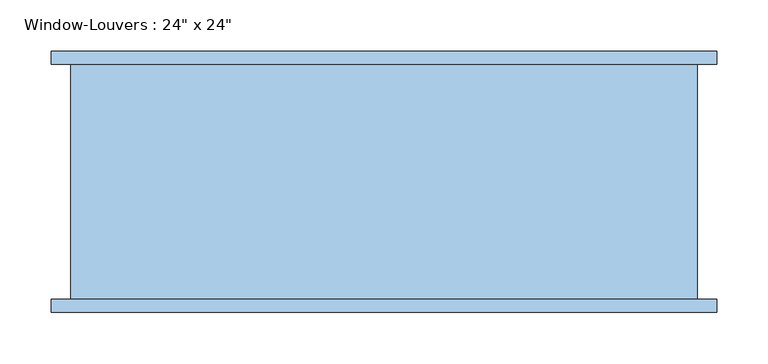
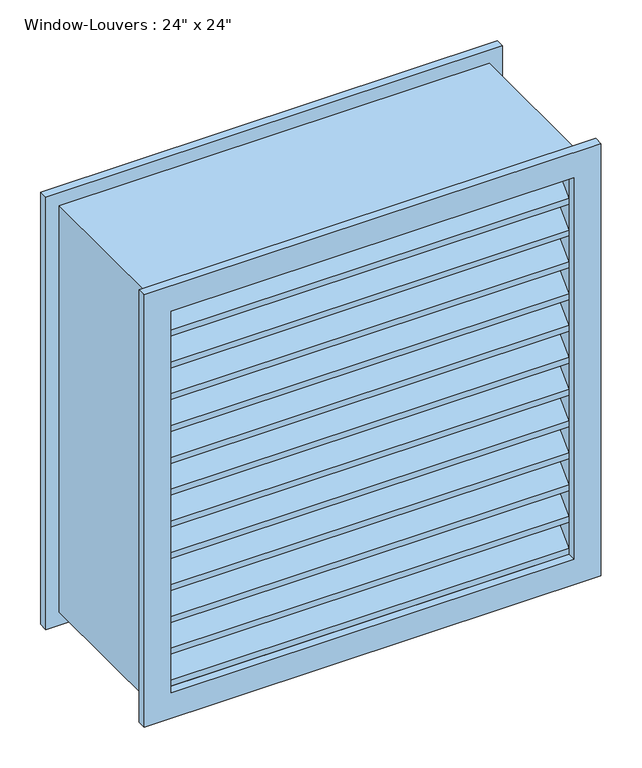
"""IFC4 building model written with IfcOpenShell, lengths in millimetres: window geometry."""

from ifc_helpers import new_model, si_unit, frame, origin, place, context, project, spatial, polyline, outline, extrude, source, transform, mapped, element, save


def window_407d3824(model_context):
    return source(origin(), model_context, "Body", "SweptSolid", [
        extrude(outline(polyline([(-107.95, 1419.1754778), (-69.85, 1457.2754778), (-31.75, 1419.1754778), (-31.75, 1410.1952217), (-69.85, 1448.2952217), (-107.95, 1410.1952217), (-107.95, 1419.1754778)])), frame((-285.75, 0.0, 0.0), z_axis=(1.0, 0.0, 0.0), x_axis=(0.0, 1.0, 0.0)), (0.0, 0.0, 1.0), 571.5),
        extrude(outline(polyline([(-107.95, 1371.5009557), (-69.85, 1409.6009557), (-31.75, 1371.5009557), (-31.75, 1362.5206995), (-69.85, 1400.6206995), (-107.95, 1362.5206995), (-107.95, 1371.5009557)])), frame((-285.75, 0.0, 0.0), z_axis=(1.0, 0.0, 0.0), x_axis=(0.0, 1.0, 0.0)), (0.0, 0.0, 1.0), 571.5),
        extrude(outline(polyline([(-107.95, 1323.8264335), (-69.85, 1361.9264335), (-31.75, 1323.8264335), (-31.75, 1314.8461774), (-69.85, 1352.9461774), (-107.95, 1314.8461774), (-107.95, 1323.8264335)])), frame((-285.75, 0.0, 0.0), z_axis=(1.0, 0.0, 0.0), x_axis=(0.0, 1.0, 0.0)), (0.0, 0.0, 1.0), 571.5),
        extrude(outline(polyline([(-107.95, 1276.1519113), (-69.85, 1314.2519113), (-31.75, 1276.1519113), (-31.75, 1267.1716552), (-69.85, 1305.2716552), (-107.95, 1267.1716552), (-107.95, 1276.1519113)])), frame((-285.75, 0.0, 0.0), z_axis=(1.0, 0.0, 0.0), x_axis=(0.0, 1.0, 0.0)), (0.0, 0.0, 1.0), 571.5),
        extrude(outline(polyline([(-107.95, 1228.4773891), (-69.85, 1266.5773891), (-31.75, 1228.4773891), (-31.75, 1219.497133), (-69.85, 1257.597133), (-107.95, 1219.497133), (-107.95, 1228.4773891)])), frame((-285.75, 0.0, 0.0), z_axis=(1.0, 0.0, 0.0), x_axis=(0.0, 1.0, 0.0)), (0.0, 0.0, 1.0), 571.5),
        extrude(outline(polyline([(-107.95, 1180.802867), (-69.85, 1218.902867), (-31.75, 1180.802867), (-31.75, 1171.8226109), (-69.85, 1209.9226109), (-107.95, 1171.8226109), (-107.95, 1180.802867)])), frame((-285.75, 0.0, 0.0), z_axis=(1.0, 0.0, 0.0), x_axis=(0.0, 1.0, 0.0)), (0.0, 0.0, 1.0), 571.5),
        extrude(outline(polyline([(-107.95, 1133.1283448), (-69.85, 1171.2283448), (-31.75, 1133.1283448), (-31.75, 1124.1480887), (-69.85, 1162.2480887), (-107.95, 1124.1480887), (-107.95, 1133.1283448)])), frame((-285.75, 0.0, 0.0), z_axis=(1.0, 0.0, 0.0), x_axis=(0.0, 1.0, 0.0)), (0.0, 0.0, 1.0), 571.5),
        extrude(outline(polyline([(-107.95, 1085.4538226), (-69.85, 1123.5538226), (-31.75, 1085.4538226), (-31.75, 1076.4735665), (-69.85, 1114.5735665), (-107.95, 1076.4735665), (-107.95, 1085.4538226)])), frame((-285.75, 0.0, 0.0), z_axis=(1.0, 0.0, 0.0), x_axis=(0.0, 1.0, 0.0)), (0.0, 0.0, 1.0), 571.5),
        extrude(outline(polyline([(-107.95, 1037.7793005), (-69.85, 1075.8793005), (-31.75, 1037.7793005), (-31.75, 1028.7990443), (-69.85, 1066.8990443), (-107.95, 1028.7990443), (-107.95, 1037.7793005)])), frame((-285.75, 0.0, 0.0), z_axis=(1.0, 0.0, 0.0), x_axis=(0.0, 1.0, 0.0)), (0.0, 0.0, 1.0), 571.5),
        extrude(outline(polyline([(-107.95, 990.1047783), (-69.85, 1028.2047783), (-31.75, 990.1047783), (-31.75, 981.1245222), (-69.85, 1019.2245222), (-107.95, 981.1245222), (-107.95, 990.1047783)])), frame((-285.75, 0.0, 0.0), z_axis=(1.0, 0.0, 0.0), x_axis=(0.0, 1.0, 0.0)), (0.0, 0.0, 1.0), 571.5),
        extrude(outline(polyline([(-107.95, 1466.85), (-69.85, 1504.95), (-31.75, 1466.85), (-31.75, 1457.8697439), (-69.85, 1495.9697439), (-107.95, 1457.8697439), (-107.95, 1466.85)])), frame((-285.75, 0.0, 0.0), z_axis=(1.0, 0.0, 0.0), x_axis=(0.0, 1.0, 0.0)), (0.0, 0.0, 1.0), 571.5),
        extrude(outline(polyline([(-107.95, 942.4302561), (-69.85, 980.5302561), (-31.75, 942.4302561), (-31.75, 933.45), (-69.85, 971.55), (-107.95, 933.45), (-107.95, 942.4302561)])), frame((-285.75, 0.0, 0.0), z_axis=(1.0, 0.0, 0.0), x_axis=(0.0, 1.0, 0.0)), (0.0, 0.0, 1.0), 571.5),
        extrude(outline(polyline([(1524.0, 304.8), (1524.0, -304.8), (914.4, -304.8), (914.4, 304.8), (1524.0, 304.8)]), holes=[polyline([(1504.95, 285.75), (933.45, 285.75), (933.45, -285.75), (1504.95, -285.75), (1504.95, 285.75)])]), frame((0.0, -107.95, 0.0), z_axis=(0.0, 1.0, 0.0), x_axis=(0.0, 0.0, 1.0)), (0.0, 0.0, 1.0), 228.6),
        extrude(outline(polyline([(1543.05, 323.85), (1543.05, -323.85), (895.35, -323.85), (895.35, 323.85), (1543.05, 323.85)]), holes=[polyline([(1504.95, 285.75), (933.45, 285.75), (933.45, -285.75), (1504.95, -285.75), (1504.95, 285.75)])]), frame((0.0, 120.65, 0.0), z_axis=(0.0, 1.0, 0.0), x_axis=(0.0, 0.0, 1.0)), (0.0, 0.0, 1.0), 12.7),
        extrude(outline(polyline([(1543.05, -323.85), (895.35, -323.85), (895.35, 323.85), (1543.05, 323.85), (1543.05, -323.85)]), holes=[polyline([(1504.95, -285.75), (1504.95, 285.75), (933.45, 285.75), (933.45, -285.75), (1504.95, -285.75)])]), frame((0.0, -120.65, 0.0), z_axis=(0.0, 1.0, 0.0), x_axis=(0.0, 0.0, 1.0)), (0.0, 0.0, 1.0), 12.7),
    ])


if __name__ == "__main__":
    model = new_model("IFC4")
    model_context = context("Model", 3, world=origin())
    ifc_project = project(units=[si_unit("LENGTHUNIT", "METRE", prefix="MILLI")], contexts=[model_context])
    site = spatial("IfcSite", under=ifc_project)
    building = spatial("IfcBuilding", under=site)
    placement = place(None, origin())
    window_shape = window_407d3824(model_context)
    element("IfcWindow", 1, ObjectType="Window-Louvers : 24\" x 24\"", at=placement, inside=building, context=model_context, shape_type="MappedRepresentation", body=[
        mapped(window_shape, transform((0.0, 0.0, 0.0), x_axis=(1.0, 0.0, 0.0), y_axis=(0.0, 1.0, 0.0), z_axis=(0.0, 0.0, 1.0))),
    ])
    save(model, "model.ifc")

# Revit data of these elements
# Type "Window-Louvers : 24\" x 24\""
#   Type Mark = "18"
#   Construction Type Id = "GSP4R"
#   Assembly Code = "B20"
#   Analytic Construction = "1/8 in Pilkington single glazing"
#   Visual Light Transmittance = 0.9
#   Thermal Resistance (R) = 1.53941 (h·ft²·°F)/BTU
#   Solar Heat Gain Coefficient = 0.78
#   Max Height = 1' - 11.74264"
#   Height = 2' - 0"
#   Heat Transfer Coefficient (U) = 0.6496 BTU/(h·ft²·°F)
#   Blade Width [instance default] = 1' - 10 1/2"
#   Blade Vertical Thickness = 0' - 0.35355"
#   Blade Thickness = 0' - 0 1/4"
#   Blade Spacing = 0' - 1 1/2"
#   Blade Height = 0' - 1.85355"
#   Blade Depth = 0' - 3"
#   Blade Angle = 45.00°
#   Default Sill Height = 3' - 0"
#   Trim Projection_Exterior = 0' - 0 1/2"
#   Trim Projection_Interior = 0' - 0 1/2"
#   Trim Width_Exterior = 0' - 1 1/2"
#   Trim Width_Interior = 0' - 1 1/2"
#   Width = 2' - 0"
#   Max Blade Count = 12
#   Define Thermal Properties by = 1
#   Blade Count = 12
#   Frame Material = Birch
#   Louver Material = Birch
#   Trim Exterior Material = Birch
#   Trim Interior Material = Birch
#   Wall Closure = (empty or 0)
# Element 1 (IfcWindow, "Window-Louvers : 24\" x 24\"")
#   Materials on its faces: "Birch"
# Materials
#   "Birch": class "Wood", colour RGB 224 178 126, transparency 0, Description = "Betula Alleghaniensis", Cost = 0
